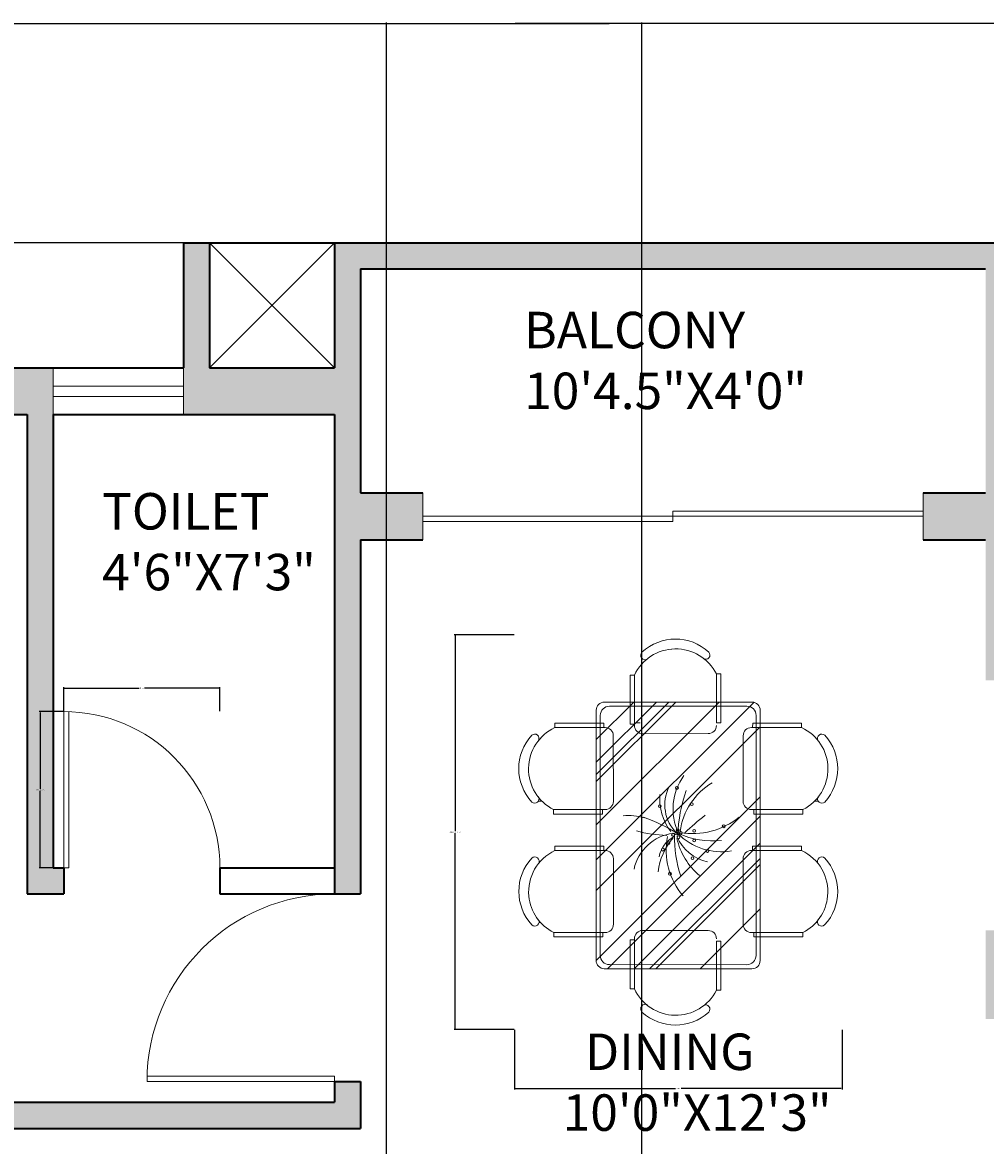
# Model space of a CAD drawing. Units: inches. Extents: x 2540 to 3167, y 3083 to 4007.
# Tile 13 of 15: x 2741 to 2926, y 3791 to 4007. Entities that reach past the tile are written whole.
import ezdxf

# ---------------------------------------------------------------- set-up
doc = ezdxf.new("R2010")
doc.units = ezdxf.units.IN
for name, color, linetype, lineweight in [('A-ANNO-DIMS', 2, 'Continuous', 18), ('A-AREA-IDEN', 7, 'Continuous', 18), ('A-DOOR', 4, 'Continuous', 18), ('A-FLOR-OPEN', 8, 'Continuous', 13), ('A-FURN', 8, 'Continuous', 13), ('A-GLAZ', 4, 'Continuous', 18)]:
    doc.layers.add(name, color=color, linetype=linetype, lineweight=lineweight)
doc.layers.add('A-WALL', color=143, linetype='Continuous', lineweight=35, true_color=0x7aafdf)
doc.layers.add('A-WALL-PATT', color=143, linetype='Continuous', lineweight=13, true_color=0x7aafdf)
doc.styles.get("Standard").update_dxf_attribs({"font": 'arial.ttf'})
doc.dimstyles.get("Standard").update_dxf_attribs({"dimtxt": 0.18, "dimasz": 0.18, "dimexe": 0.18, "dimexo": 0.0625, "dimgap": 0.09, "dimtad": 0, "dimtih": 1, "dimtoh": 1, "dimdec": 4, "dimzin": 0, "dimdsep": 46, "dimtxsty": 'Standard', "dimcen": 0.09, "dimadec": 0, "dimazin": 0, "dimtfac": 1, "dimtdec": 4, "dimtofl": 0, "dimtmove": 0, "dimatfit": 3, "dimfxl": 1, "dimtolj": 1, "dimtzin": 0, "dimarcsym": 0})

# ---------------------------------------------------------------- blocks, each defined once
blk = doc.blocks.new('A$C6327331B')
for p, q in [((790.8, 678.3), (790.8, 696.4)), ((790.8, 678.3), (790.8, 696.4)), ((1381.3, 692.8), (1381.3, 686.2)), ((1381.3, 692.8), (1381.3, 686.2)), ((410.1, 615.8), (410, 377)), ((410.1, 615.8), (410, 377)), ((431.6, 615.8), (410.1, 615.8)), ((431.6, 615.8), (410.1, 615.8)), ((431.4, 376.9), (431.6, 615.8)), ((431.4, 376.9), (431.6, 615.8)), ((831.4, 382.9), (831.6, 621.7)), ((831.4, 382.9), (831.6, 621.7)), ((831.6, 621.7), (853, 621.7)), ((831.6, 621.7), (853, 621.7)), ((853, 621.7), (852.9, 382.9)), ((853, 621.7), (852.9, 382.9)), ((1009.3, 615.5), (1009.2, 376.7)), ((1009.3, 615.5), (1009.2, 376.7)), ((1030.7, 615.5), (1009.3, 615.5)), ((1030.7, 615.5), (1009.3, 615.5)), ((1030.6, 376.6), (1030.7, 615.5)), ((1030.6, 376.6), (1030.7, 615.5)), ((1430.6, 382.6), (1430.7, 621.4)), ((1430.6, 382.6), (1430.7, 621.4)), ((1430.7, 621.4), (1452.2, 621.4)), ((1430.7, 621.4), (1452.2, 621.4)), ((1452.2, 621.4), (1452, 382.6)), ((1452.2, 621.4), (1452, 382.6)), ((431.5, 571.8), (431.4, 370.8)), ((431.5, 571.8), (431.4, 370.8)), ((831.4, 370.6), (831.5, 571.6)), ((831.4, 370.6), (831.5, 571.6)), ((1030.7, 571.5), (1030.6, 370.5)), ((1030.7, 571.5), (1030.6, 370.5)), ((1430.6, 370.3), (1430.7, 571.3)), ((1430.6, 370.3), (1430.7, 571.3)), ((347.5, 414), (831.5, 413.8)), ((347.5, 414), (831.5, 413.8)), ((372.5, 394), (831.4, 393.8)), ((372.5, 394), (1009.2, 393.7)), ((1226.3, -386.4), (428, 414)), ((1226.3, -386.4), (428, 414)), ((1567.1, -386.6), (768.8, 413.8)), ((1567.1, -386.6), (768.8, 413.8)), ((831.5, 413.8), (1567.5, 413.4)), ((1607.1, -331.3), (864.1, 413.8)), ((1607.1, -331.3), (864.1, 413.8)), ((1607.2, -200.8), (994.4, 413.7)), ((1607.2, -200.8), (994.4, 413.7)), ((1009.2, 413.7), (1567.5, 413.4)), ((1009.2, 393.7), (1542.5, 393.4)), ((1607.2, -125.5), (1069.5, 413.7)), ((1607.2, -125.5), (1069.5, 413.7)), ((1607.2, -95.4), (1099.6, 413.6)), ((1607.2, -95.4), (1099.6, 413.6)), ((1607.3, 120.5), (1315.1, 413.5)), ((1607.3, 120.5), (1315.1, 413.5)), ((1415.7, 413.4), (1415.7, 413.5)), ((1415.7, 413.4), (1415.7, 413.5)), ((307.1, -346), (307.5, 374)), ((307.1, -346), (307.5, 374)), ((1075.9, -386.3), (308.5, 383.1)), ((1075.9, -386.3), (308.5, 383.1)), ((327.1, -321), (327.5, 349)), ((410, 377), (431.4, 376.9)), ((410, 377), (431.4, 376.9)), ((471.4, 330.8), (791.4, 330.6)), ((471.4, 330.8), (791.4, 330.6)), ((852.9, 382.9), (831.4, 382.9)), ((852.9, 382.9), (831.4, 382.9)), ((1009.2, 376.7), (1030.6, 376.6)), ((1009.2, 376.7), (1030.6, 376.6)), ((1070.6, 330.5), (1390.6, 330.3)), ((1070.6, 330.5), (1390.6, 330.3)), ((1452, 382.6), (1430.6, 382.6)), ((1452, 382.6), (1430.6, 382.6)), ((1587.5, 348.4), (1587.1, -321.6)), ((1607.5, 373.4), (1607.1, -346.6)), ((1607.5, 373.4), (1607.1, -346.6)), ((169.9, 221.5), (408.7, 221.6)), ((169.9, 221.5), (408.7, 221.6)), ((169.9, 200.1), (169.9, 221.5)), ((169.9, 200.1), (169.9, 221.5)), ((408.7, 221.6), (408.7, 200.2)), ((408.7, 221.6), (408.7, 200.2)), ((1473.3, 221.6), (1473.3, 200.2)), ((1473.3, 221.6), (1473.3, 200.2)), ((1712.1, 221.5), (1473.3, 221.6)), ((1712.1, 221.5), (1473.3, 221.6)), ((1712.1, 200.1), (1712.1, 221.5)), ((1712.1, 200.1), (1712.1, 221.5)), ((408.7, 200.2), (169.9, 200.1)), ((408.7, 200.2), (169.9, 200.1)), ((905.5, -386.3), (307.4, 213.5)), ((905.5, -386.3), (307.4, 213.5)), ((1473.3, 200.2), (1712.1, 200.1)), ((1473.3, 200.2), (1712.1, 200.1)), ((461.2, -159.8), (461, 160.2)), ((461.2, -159.8), (461, 160.2)), ((1420.8, -159.8), (1420.9, 160.2)), ((1420.8, -159.8), (1420.9, 160.2)), ((695.1, -386.2), (307.3, 2.7)), ((695.1, -386.2), (307.3, 2.7)), ((44.6, -20.2), (44.5, -20.1)), ((44.6, -20.2), (44.5, -20.1)), ((660, -386.1), (307.3, -32.5)), ((660, -386.1), (307.3, -32.5)), ((1837.4, -20.2), (1837.5, -20.1)), ((1837.4, -20.2), (1837.5, -20.1)), ((599.8, -386.1), (307.2, -92.7)), ((599.8, -386.1), (307.2, -92.7)), ((415.1, -199.8), (176.2, -199.9)), ((415.1, -199.8), (176.2, -199.9)), ((176.2, -199.9), (176.2, -221.3)), ((176.2, -199.9), (176.2, -221.3)), ((220.2, -199.9), (421.2, -199.8)), ((220.2, -199.9), (421.2, -199.8)), ((489.6, -386), (307.2, -203.2)), ((489.6, -386), (307.2, -203.2)), ((408.7, -193.6), (408.7, -172.1)), ((408.7, -193.6), (408.7, -172.1)), ((415.1, -221.2), (415.1, -199.8)), ((415.1, -221.2), (415.1, -199.8)), ((1661.8, -199.9), (1460.8, -199.8)), ((1661.8, -199.9), (1460.8, -199.8)), ((1466.9, -221.2), (1466.9, -199.8)), ((1466.9, -221.2), (1466.9, -199.8)), ((1466.9, -199.8), (1705.7, -199.9)), ((1466.9, -199.8), (1705.7, -199.9)), ((1705.7, -199.9), (1705.7, -221.3)), ((1705.7, -199.9), (1705.7, -221.3)), ((176.2, -221.3), (415.1, -221.2)), ((176.2, -221.3), (415.1, -221.2)), ((1705.7, -221.3), (1466.9, -221.2)), ((1705.7, -221.3), (1466.9, -221.2)), ((471.4, -302.7), (791.4, -302.5)), ((471.4, -302.7), (791.4, -302.5)), ((1070.6, -302.4), (1390.6, -302.2)), ((1070.6, -302.4), (1390.6, -302.2)), ((1542.1, -366.6), (372.1, -366)), ((410.1, -587.7), (410, -348.9)), ((410.1, -587.7), (410, -348.9)), ((410, -348.9), (431.4, -348.9)), ((410, -348.9), (431.4, -348.9)), ((431.5, -543.7), (431.4, -342.7)), ((431.5, -543.7), (431.4, -342.7)), ((431.4, -348.9), (431.6, -587.7)), ((431.4, -348.9), (431.6, -587.7)), ((831.4, -342.5), (831.5, -543.5)), ((831.4, -342.5), (831.5, -543.5)), ((831.4, -354.8), (831.6, -593.6)), ((831.4, -354.8), (831.6, -593.6)), ((852.9, -354.8), (831.4, -354.8)), ((852.9, -354.8), (831.4, -354.8)), ((853, -593.6), (852.9, -354.8)), ((853, -593.6), (852.9, -354.8)), ((1009.2, -348.6), (1030.6, -348.5)), ((1009.2, -348.6), (1030.6, -348.5)), ((1009.3, -587.4), (1009.2, -348.6)), ((1009.3, -587.4), (1009.2, -348.6)), ((1030.7, -543.4), (1030.6, -342.4)), ((1030.7, -543.4), (1030.6, -342.4)), ((1030.6, -348.5), (1030.7, -587.4)), ((1030.6, -348.5), (1030.7, -587.4)), ((1430.6, -342.2), (1430.7, -543.2)), ((1430.6, -342.2), (1430.7, -543.2)), ((1430.6, -354.5), (1430.7, -593.3)), ((1430.6, -354.5), (1430.7, -593.3)), ((1452, -354.5), (1430.6, -354.5)), ((1452, -354.5), (1430.6, -354.5)), ((1452.2, -593.3), (1452, -354.5)), ((1452.2, -593.3), (1452, -354.5)), ((1567.1, -386.6), (347.1, -386)), ((1567.1, -386.6), (347.1, -386)), ((831.5, -385.7), (864.1, -385.7)), ((831.5, -385.7), (864.1, -385.7)), ((1415.7, -385.3), (1415.7, -385.4)), ((1415.7, -385.3), (1415.7, -385.4)), ((431.6, -587.7), (410.1, -587.7)), ((431.6, -587.7), (410.1, -587.7)), ((831.6, -593.6), (853, -593.6)), ((831.6, -593.6), (853, -593.6)), ((1030.7, -587.4), (1009.3, -587.4)), ((1030.7, -587.4), (1009.3, -587.4)), ((1430.7, -593.3), (1452.2, -593.3)), ((1430.7, -593.3), (1452.2, -593.3)), ((790.8, -650.2), (790.8, -668.4)), ((790.8, -650.2), (790.8, -668.4)), ((1381.3, -664.7), (1381.3, -658.1)), ((1381.3, -664.7), (1381.3, -658.1))]:
    blk.add_line(p, q)
for centre, radius, start, end in [((631.5, 550.5), 241.3, 47.4691, 132.4721), ((631.5, 550.5), 241.3, 47.4691, 132.4721), ((1230.7, 550.2), 241.3, 47.4691, 132.4721), ((1230.7, 550.2), 241.3, 47.4691, 132.4721), ((633, 521.6), 222.4, 26.7656, 154.9369), ((633, 521.6), 222.4, 26.7656, 154.9369), ((484.3, 714.2), 21.2, 137.6497, 300.3412), ((484.3, 714.2), 21.2, 137.6497, 300.3412), ((779, 714), 21.2, 239.6, 42.2915), ((779, 714), 21.2, 239.6, 42.2915), ((1232.2, 521.3), 222.4, 84.4265, 154.9369), ((1232.2, 521.3), 222.4, 84.4265, 154.9369), ((1083.4, 713.9), 21.2, 137.6497, 300.3412), ((1083.4, 713.9), 21.2, 137.6497, 300.3412), ((1232.2, 521.3), 222.4, 26.7656, 84.4265), ((1232.2, 521.3), 222.4, 26.7656, 84.4265), ((1378.1, 713.7), 21.2, 239.6, 42.2915), ((1378.1, 713.7), 21.2, 239.6, 42.2915), ((347.5, 374), 40, 89.9706, 179.9706), ((347.5, 374), 40, 89.9706, 179.9706), ((372.5, 349), 45, 89.9706, 179.9706), ((1542.5, 348.4), 45, 359.9706, 89.9706), ((1567.5, 373.4), 40, 359.9706, 89.9706), ((1567.5, 373.4), 40, 359.9706, 89.9706), ((471.4, 370.8), 40, 179.9706, 269.9706), ((471.4, 370.8), 40, 179.9706, 269.9706), ((791.4, 370.6), 40, 269.9706, 359.9706), ((791.4, 370.6), 40, 269.9706, 359.9706), ((1070.6, 370.5), 40, 179.9706, 269.9706), ((1070.6, 370.5), 40, 179.9706, 269.9706), ((1390.6, 370.3), 40, 269.9706, 359.9706), ((1390.6, 370.3), 40, 269.9706, 359.9706), ((574.1, 79.9), 374.6, 351.2496, 38.2333), ((912.6, 235.7), 6.91, 0, 180), ((912.6, 235.7), 6.91, 180, 0), ((737.8, 225), 299.2, 314.4861, 9.3762), ((586.4, 182.9), 398.1, 335.0888, 5.9637), ((270.2, 1.6), 222.4, 116.8244, 244.9957), ((270.2, 1.6), 222.4, 116.8244, 244.9957), ((77.6, 147.4), 21.2, 329.6588, 132.3503), ((77.6, 147.4), 21.2, 329.6588, 132.3503), ((421, 160.2), 40, 0.0294, 90.0294), ((421, 160.2), 40, 0.0294, 90.0294), ((983.2, 350.8), 331, 211.315, 262.1378), ((1460.9, 160.2), 40, 89.9706, 179.9706), ((1460.9, 160.2), 40, 89.9706, 179.9706), ((1611.7, 1.6), 222.4, 295.0043, 63.1756), ((1611.7, 1.6), 222.4, 295.0043, 63.1756), ((1804.4, 147.4), 21.2, 47.6497, 210.3412), ((1804.4, 147.4), 21.2, 47.6497, 210.3412), ((241.3, 0.1), 241.3, 137.5279, 222.5309), ((2460.3, 1443.6), 2062.1, 219.0488, 222.6799), ((873.8, 207.8), 219.3, 294.0956, 346.2953), ((897.1, 334.6), 335.6, 283.0452, 319.7766), ((1033, 155.9), 6.91, 0, 180), ((1033, 155.9), 6.91, 180, 0), ((1640.7, 0.1), 241.3, 317.4691, 42.4721), ((1640.7, 0.1), 241.3, 317.4691, 42.4721), ((805, 79.9), 6.91, 0, 180), ((805, 79.9), 6.91, 180, 0), ((934.8, 91.3), 6.91, 0, 180), ((934.8, 91.3), 6.91, 180, 0), ((982.3, 91.3), 6.91, 0, 180), ((982.3, 91.3), 6.91, 180, 0), ((1067.8, 83.7), 6.91, 0, 180), ((1067.8, 83.7), 6.91, 180, 0), ((826.9, 258.5), 270.1, 233.3231, 295.7633), ((725.8, 7.7), 6.91, 0, 180), ((725.8, 7.7), 6.91, 180, 0), ((807.8, 143), 194.5, 242.9909, 315.9102), ((985.1, 750.7), 739.8, 250.5249, 267.8244), ((1747.6, -469.5), 933.6, 148.9873, 160.361), ((931.7, 11.5), 6.91, 0, 180), ((931.7, 11.5), 6.91, 180, 0), ((944.3, 26.7), 6.91, 0, 180), ((944.3, 26.7), 6.91, 180, 0), ((947.5, 3.9), 6.91, 0, 180), ((947.5, 3.9), 6.91, 180, 0), ((970.7, 574.8), 578.8, 268.3286, 288.729), ((966.5, 15.3), 6.91, 0, 180), ((966.5, 15.3), 6.91, 180, 0), ((1030.3, 292.7), 337.4, 258.5516, 310.9815), ((776.7, 191.6), 268.2, 265.8741, 306.9558), ((392.7, -33), 564.4, 343.8561, 359.1105), ((953.8, -11.3), 6.91, 0, 180), ((953.8, -11.3), 6.91, 180, 0), ((1167.7, 15.7), 221.9, 186.9904, 258.0284), ((1090.6, 62.7), 145.4, 208.8901, 258.4579), ((1166.2, 212.9), 298.2, 228.7581, 263.8624), ((995, -34.1), 6.91, 0, 180), ((995, -34.1), 6.91, 180, 0), ((1026.7, -60.7), 6.91, 0, 180), ((1143.8, -26.5), 6.91, 0, 180), ((1143.8, -26.5), 6.91, 180, 0), ((814.5, -75.9), 6.91, 0, 180), ((814.5, -75.9), 6.91, 180, 0), ((1026.7, -60.7), 6.91, 180, 0), ((79, -146.7), 22.5, 226.3776, 29.8882), ((79, -146.7), 22.5, 226.3776, 29.8882), ((421.2, -159.8), 40, 270.0294, 0.0294), ((421.2, -159.8), 40, 270.0294, 0.0294), ((1112.9, -226), 252.6, 162.9456, 186.4814), ((1460.8, -159.8), 40, 179.9706, 269.9706), ((1460.8, -159.8), 40, 179.9706, 269.9706), ((1803, -146.7), 22.5, 150.1118, 313.6224), ((1803, -146.7), 22.5, 150.1118, 313.6224), ((372.1, -321), 45, 179.9706, 269.9706), ((471.4, -342.7), 40, 90.0294, 180.0294), ((471.4, -342.7), 40, 90.0294, 180.0294), ((791.4, -342.5), 40, 0.0294, 90.0294), ((791.4, -342.5), 40, 0.0294, 90.0294), ((1070.6, -342.4), 40, 90.0294, 180.0294), ((1070.6, -342.4), 40, 90.0294, 180.0294), ((1390.6, -342.2), 40, 0.0294, 90.0294), ((1390.6, -342.2), 40, 0.0294, 90.0294), ((1542.1, -321.6), 45, 269.9706, 359.9706), ((347.1, -346), 40, 179.9706, 269.9706), ((347.1, -346), 40, 179.9706, 269.9706), ((1567.1, -346.6), 40, 269.9706, 359.9706), ((1567.1, -346.6), 40, 269.9706, 359.9706), ((633, -493.5), 222.4, 205.0631, 333.2344), ((633, -493.5), 222.4, 205.0631, 333.2344), ((1232.2, -493.2), 222.4, 205.0631, 275.5735), ((1232.2, -493.2), 222.4, 205.0631, 275.5735), ((1232.2, -493.2), 222.4, 275.5735, 333.2344), ((1232.2, -493.2), 222.4, 275.5735, 333.2344), ((484.3, -686.1), 21.2, 59.6588, 222.3503), ((484.3, -686.1), 21.2, 59.6588, 222.3503), ((631.5, -522.4), 241.3, 227.5279, 312.5309), ((631.5, -522.4), 241.3, 227.5279, 312.5309), ((779, -686), 21.2, 317.7085, 120.4), ((779, -686), 21.2, 317.7085, 120.4), ((1083.4, -685.8), 21.2, 59.6588, 222.3503), ((1083.4, -685.8), 21.2, 59.6588, 222.3503), ((1230.7, -522.1), 241.3, 227.5279, 312.5309), ((1230.7, -522.1), 241.3, 227.5279, 312.5309), ((1378.1, -685.6), 21.2, 317.7085, 120.4), ((1378.1, -685.6), 21.2, 317.7085, 120.4)]:
    blk.add_arc(centre, radius, start, end)
at = {"width": 0.8, "flags": 9}
for tag in ['XSIZE', 'YSIZE']:
    blk.add_attdef(tag, (945.2, 11.4), '', height=0.23, rotation=180, dxfattribs=at)
blk = doc.blocks.new('DOOR-SWING-36IN')
for p, q in [((36, 0), (0, 0)), ((36, 1), (0.01, 1)), ((36, 1), (36, 0))]:
    blk.add_line(p, q)
blk.add_arc((36, 0), 36, 90, 180)
blk = doc.blocks.new('DOOR-SWING-30IN')
for p, q in [((0, 0), (0, 30)), ((1, 0), (1, 29.98)), ((0, 0), (1, 0))]:
    blk.add_line(p, q)
blk.add_arc((0, 0), 30, 0, 90)
blk = doc.blocks.new('OPENING-CROSS-24IN')
for p, q in [((24, 24), (0, 0)), ((0, 24), (24, 0))]:
    blk.add_line(p, q)
blk = doc.blocks.new('*D21')
at = {"layer": 'A-ANNO-DIMS', "color": 0, "lineweight": -2, "transparency": 16777216}
for p, q in [((2748.45, 3874.71), (2743.83, 3874.71)), ((2744.01, 3874.53), (2744.01, 3859.9)), ((2744.01, 3844.89), (2744.01, 3859.53)), ((2748.45, 3844.71), (2743.83, 3844.71))]:
    blk.add_line(p, q, dxfattribs=at)
at = {"layer": 'A-ANNO-DIMS', "color": 0, "transparency": 16777216}
for points in [[(2743.98, 3874.53), (2744.04, 3874.53), (2744.01, 3874.71)], [(2743.98, 3844.89), (2744.04, 3844.89), (2744.01, 3844.71)]]:
    blk.add_solid(points, dxfattribs=at)
at = {"layer": 'Defpoints', "color": 0, "transparency": 16777216}
for p in [(2744.01, 3874.71), (2748.51, 3874.71), (2748.51, 3844.71)]:
    blk.add_point(p, dxfattribs=at)
at = {"layer": 'A-ANNO-DIMS', "color": 0, "transparency": 16777216, "insert": (2744.01, 3859.71), "char_height": 0.18, "attachment_point": 5}
blk.add_mtext('\\A1;DOOR 30 TYP.', dxfattribs=at)
blk = doc.blocks.new('*D22')
at = {"layer": 'A-ANNO-DIMS', "color": 0, "lineweight": -2, "transparency": 16777216}
for p, q in [((2748.51, 3874.78), (2748.51, 3879.39)), ((2748.69, 3879.21), (2762.98, 3879.21)), ((2778.33, 3879.21), (2764.04, 3879.21)), ((2778.51, 3874.78), (2778.51, 3879.39))]:
    blk.add_line(p, q, dxfattribs=at)
at = {"layer": 'A-ANNO-DIMS', "color": 0, "transparency": 16777216}
for points in [[(2748.69, 3879.24), (2748.69, 3879.18), (2748.51, 3879.21)], [(2778.33, 3879.24), (2778.33, 3879.18), (2778.51, 3879.21)]]:
    blk.add_solid(points, dxfattribs=at)
at = {"layer": 'Defpoints', "color": 0, "transparency": 16777216}
for p in [(2778.51, 3879.21), (2748.51, 3874.71), (2778.51, 3874.71)]:
    blk.add_point(p, dxfattribs=at)
at = {"layer": 'A-ANNO-DIMS', "color": 0, "transparency": 16777216, "insert": (2763.51, 3879.21), "char_height": 0.18, "attachment_point": 5}
blk.add_mtext('\\A1;30 TYP.', dxfattribs=at)
blk = doc.blocks.new('*D37')
at = {"layer": 'A-ANNO-DIMS', "color": 0, "lineweight": -2, "transparency": 16777216}
for p, q in [((2834.99, 3889.47), (2823.51, 3889.47)), ((2823.69, 3889.29), (2823.69, 3851.77)), ((2823.69, 3813.89), (2823.69, 3851.4)), ((2834.99, 3813.71), (2823.51, 3813.71))]:
    blk.add_line(p, q, dxfattribs=at)
at = {"layer": 'A-ANNO-DIMS', "color": 0, "transparency": 16777216}
for points in [[(2823.66, 3889.29), (2823.72, 3889.29), (2823.69, 3889.47)], [(2823.66, 3813.89), (2823.72, 3813.89), (2823.69, 3813.71)]]:
    blk.add_solid(points, dxfattribs=at)
at = {"layer": 'Defpoints', "color": 0, "transparency": 16777216}
for p in [(2835.06, 3889.47), (2823.69, 3813.71), (2835.06, 3813.71)]:
    blk.add_point(p, dxfattribs=at)
at = {"layer": 'A-ANNO-DIMS', "color": 0, "transparency": 16777216, "insert": (2823.69, 3851.59), "char_height": 0.18, "attachment_point": 5}
blk.add_mtext('\\A1;DINING SET 76 TYP.', dxfattribs=at)
blk = doc.blocks.new('*D38')
at = {"layer": 'A-ANNO-DIMS', "color": 0, "lineweight": -2, "transparency": 16777216}
for p, q in [((2835.06, 3813.64), (2835.06, 3802.16)), ((2897.96, 3813.64), (2897.96, 3802.16)), ((2835.24, 3802.34), (2865.98, 3802.34)), ((2897.78, 3802.34), (2867.04, 3802.34))]:
    blk.add_line(p, q, dxfattribs=at)
at = {"layer": 'A-ANNO-DIMS', "color": 0, "transparency": 16777216}
for points in [[(2835.24, 3802.37), (2835.24, 3802.31), (2835.06, 3802.34)], [(2897.78, 3802.37), (2897.78, 3802.31), (2897.96, 3802.34)]]:
    blk.add_solid(points, dxfattribs=at)
at = {"layer": 'Defpoints', "color": 0, "transparency": 16777216}
for p in [(2835.06, 3813.71), (2897.96, 3813.71), (2897.96, 3802.34)]:
    blk.add_point(p, dxfattribs=at)
at = {"layer": 'A-ANNO-DIMS', "color": 0, "transparency": 16777216, "insert": (2866.51, 3802.34), "char_height": 0.18, "attachment_point": 5}
blk.add_mtext('\\A1;63 TYP.', dxfattribs=at)
blk = doc.blocks.new('*D43')
at = {"layer": 'A-ANNO-DIMS', "color": 0, "lineweight": -2, "transparency": 16777216}
for p, q in [((2582.51, 3940.78), (2582.51, 4006.99)), ((2582.69, 4006.81), (2853.22, 4006.81)), ((3124.33, 4006.81), (2853.8, 4006.81)), ((3124.51, 3940.78), (3124.51, 4006.99))]:
    blk.add_line(p, q, dxfattribs=at)
at = {"layer": 'A-ANNO-DIMS', "color": 0, "transparency": 16777216}
for points in [[(2582.69, 4006.84), (2582.69, 4006.78), (2582.51, 4006.81)], [(3124.33, 4006.84), (3124.33, 4006.78), (3124.51, 4006.81)]]:
    blk.add_solid(points, dxfattribs=at)
at = {"layer": 'Defpoints', "color": 0, "transparency": 16777216}
for p in [(3124.51, 4006.81), (2582.51, 3940.71), (3124.51, 3940.71)]:
    blk.add_point(p, dxfattribs=at)
at = {"layer": 'A-ANNO-DIMS', "color": 0, "transparency": 16777216, "insert": (2853.51, 4006.81), "char_height": 0.18, "attachment_point": 5}
blk.add_mtext('\\A1;542', dxfattribs=at)
blk = doc.blocks.new('*D44')
at = {"layer": 'A-ANNO-DIMS', "color": 0, "lineweight": -2, "transparency": 16777216}
for p, q in [((2771.45, 3964.71), (2540.23, 3964.71)), ((2540.41, 3964.53), (2540.41, 3545.4)), ((2540.41, 3125.89), (2540.41, 3545.03)), ((2810.45, 3125.71), (2540.23, 3125.71))]:
    blk.add_line(p, q, dxfattribs=at)
at = {"layer": 'A-ANNO-DIMS', "color": 0, "transparency": 16777216}
for points in [[(2540.38, 3964.53), (2540.44, 3964.53), (2540.41, 3964.71)], [(2540.38, 3125.89), (2540.44, 3125.89), (2540.41, 3125.71)]]:
    blk.add_solid(points, dxfattribs=at)
at = {"layer": 'Defpoints', "color": 0, "transparency": 16777216}
for p in [(2540.41, 3964.71), (2771.51, 3964.71), (2810.51, 3125.71)]:
    blk.add_point(p, dxfattribs=at)
at = {"layer": 'A-ANNO-DIMS', "color": 0, "transparency": 16777216, "insert": (2540.41, 3545.21), "char_height": 0.18, "attachment_point": 5}
blk.add_mtext('\\A1;839', dxfattribs=at)
blk = doc.blocks.new('*D56')
at = {"layer": 'A-ANNO-DIMS', "color": 0, "lineweight": -2, "transparency": 16777216}
for p, q in [((2810.51, 3564.78), (2810.51, 4006.99)), ((2810.69, 4006.81), (2834.79, 4006.81)), ((2859.33, 4006.81), (2835.23, 4006.81)), ((2859.51, 3564.78), (2859.51, 4006.99))]:
    blk.add_line(p, q, dxfattribs=at)
at = {"layer": 'A-ANNO-DIMS', "color": 0, "transparency": 16777216}
for points in [[(2810.69, 4006.84), (2810.69, 4006.78), (2810.51, 4006.81)], [(2859.33, 4006.84), (2859.33, 4006.78), (2859.51, 4006.81)]]:
    blk.add_solid(points, dxfattribs=at)
at = {"layer": 'Defpoints', "color": 0, "transparency": 16777216}
for p in [(2859.51, 4006.81), (2810.51, 3564.71), (2859.51, 3564.71)]:
    blk.add_point(p, dxfattribs=at)
at = {"layer": 'A-ANNO-DIMS', "color": 0, "transparency": 16777216, "insert": (2835.01, 4006.81), "char_height": 0.18, "attachment_point": 5}
blk.add_mtext('\\A1;49', dxfattribs=at)

msp = doc.modelspace()

# ---------------------------------------------------------------- hatches: boundary and pattern name
at = {"layer": 'A-WALL-PATT'}
h = msp.add_hatch(color=256, dxfattribs=at)
h.dxf.hatch_style = 1
h.paths.add_polyline_path([(2644.77, 3940.71), (2582.51, 3940.71), (2582.51, 3886.71), (2612.51, 3886.71), (2612.51, 3871.71), (2621.51, 3871.71), (2621.51, 3895.71), (2591.51, 3895.71), (2591.51, 3931.71), (2621.51, 3931.71), (2644.77, 3931.71)])
h.paths.add_polyline_path([(2746.51, 3940.71), (2716.77, 3940.71), (2716.77, 3931.71), (2741.51, 3931.71), (2741.51, 3839.71), (2748.51, 3839.71), (2748.51, 3844.71), (2746.51, 3844.71), (2746.51, 3931.71)])
h.paths.add_polyline_path([(2805.51, 3959.71), (2925.51, 3959.71), (2925.51, 3916.71), (2913.51, 3916.71), (2913.51, 3907.71), (2925.51, 3907.71), (2925.51, 3880.71), (2930.51, 3880.71), (2930.51, 3931.71), (2978.28, 3931.71), (2978.28, 3940.71), (2930.51, 3940.71), (2930.51, 3964.71), (2800.51, 3964.71), (2800.51, 3940.71), (2776.51, 3940.71), (2776.51, 3964.71), (2771.51, 3964.71), (2771.51, 3940.71), (2771.51, 3931.71), (2800.51, 3931.71), (2800.51, 3839.71), (2805.51, 3839.71), (2805.51, 3907.71), (2817.48, 3907.71), (2817.48, 3916.71), (2805.51, 3916.71)])
h.paths.add_polyline_path([(3124.51, 3940.71), (3026.28, 3940.71), (3026.28, 3931.71), (3062.51, 3931.71), (3062.51, 3924.21), (3071.51, 3924.21), (3071.51, 3931.71), (3119.51, 3931.71), (3119.51, 3832.71), (2925.51, 3832.71), (2925.51, 3815.71), (2930.51, 3815.71), (2930.51, 3827.71), (2976.51, 3827.71), (2976.51, 3773.71), (2970.51, 3773.71), (2970.51, 3768.71), (2985.51, 3768.71), (2985.51, 3773.71), (2981.51, 3773.71), (2981.51, 3827.71), (3086.51, 3827.71), (3086.51, 3812.71), (3095.51, 3812.71), (3095.51, 3827.71), (3124.51, 3827.71)])
h = msp.add_hatch(color=256, dxfattribs=at)
h.dxf.hatch_style = 1
h.paths.add_polyline_path([(2805.51, 3803.71), (2800.51, 3803.71), (2800.51, 3799.71), (2621.51, 3799.71), (2621.51, 3823.71), (2612.51, 3823.71), (2612.51, 3794.71), (2636.51, 3794.71), (2636.51, 3782.71), (2645.51, 3782.71), (2645.51, 3794.71), (2805.51, 3794.71)])
h.paths.add_polyline_path([(2810.51, 3564.71), (2868.51, 3564.71), (2868.51, 3627.71), (2872.51, 3627.71), (2872.51, 3636.71), (2864.51, 3636.71), (2864.51, 3674.71), (2797.51, 3674.71), (2797.51, 3669.71), (2801.51, 3669.71), (2801.51, 3628.63), (2806.51, 3628.63), (2806.51, 3669.71), (2859.51, 3669.71), (2859.51, 3573.71), (2806.51, 3573.71), (2806.51, 3598.63), (2801.51, 3598.63), (2801.51, 3549.71), (2645.51, 3549.71), (2645.51, 3573.71), (2636.51, 3573.71), (2636.51, 3516.71), (2645.51, 3516.71), (2645.51, 3540.71), (2801.51, 3540.71), (2801.51, 3504.71), (2801.51, 3500.71), (2806.51, 3500.71), (2806.51, 3504.71), (2859.51, 3504.71), (2859.51, 3420.71), (2806.51, 3420.71), (2806.51, 3470.71), (2801.51, 3470.71), (2801.51, 3420.71), (2797.51, 3420.71), (2797.51, 3415.71), (2864.51, 3415.71), (2864.51, 3453.71), (2868.51, 3453.71), (2868.51, 3513.71), (2810.51, 3513.71)])
h.paths.add_polyline_path([(2645.51, 3415.71), (2761.51, 3415.71), (2761.51, 3420.71), (2645.51, 3420.71), (2645.51, 3444.71), (2636.51, 3444.71), (2636.51, 3403.71), (2645.51, 3403.71)])
h.paths.add_polyline_path([(2645.51, 3307.71), (2636.51, 3307.71), (2636.51, 3295.71), (2612.51, 3295.71), (2612.51, 3149.71), (2645.51, 3149.71), (2645.51, 3158.71), (2621.51, 3158.71), (2621.51, 3290.71), (2801.51, 3290.71), (2801.51, 3286.71), (2806.51, 3286.71), (2806.51, 3295.71), (2645.51, 3295.71)])
h.paths.add_polyline_path([(2762.01, 3158.71), (2746.51, 3158.71), (2746.51, 3240.71), (2750.51, 3240.71), (2750.51, 3245.71), (2741.51, 3245.71), (2741.51, 3158.71), (2717.51, 3158.71), (2717.51, 3149.71), (2762.01, 3149.71)], flags=17)
h.paths.add_polyline_path([(2810.51, 3173.71), (2822.51, 3173.71), (2822.51, 3182.71), (2806.51, 3182.71), (2806.51, 3250.71), (2801.51, 3250.71), (2801.51, 3245.71), (2780.51, 3245.71), (2780.51, 3240.71), (2801.51, 3240.71), (2801.51, 3158.71), (2786.01, 3158.71), (2786.01, 3149.71), (2810.51, 3149.71)])
h.paths.add_polyline_path([(2931.51, 3290.71), (2935.51, 3290.71), (2935.51, 3295.71), (2926.51, 3295.71), (2926.51, 3182.71), (2910.51, 3182.71), (2910.51, 3173.71), (2922.51, 3173.71), (2922.51, 3149.71), (2987.51, 3149.71), (2987.51, 3158.71), (2931.51, 3158.71)])
h.paths.add_polyline_path([(3124.51, 3295.71), (3086.51, 3295.71), (3018.51, 3295.71), (3018.51, 3290.71), (3115.51, 3290.71), (3115.51, 3158.71), (3059.51, 3158.71), (3059.51, 3149.71), (3124.51, 3149.71)])
h.paths.add_polyline_path([(2988.51, 3295.71), (2984.51, 3295.71), (2984.51, 3349.71), (3086.51, 3349.71), (3086.51, 3320.71), (3124.51, 3320.71), (3124.51, 3354.71), (3071.51, 3354.71), (3071.51, 3358.71), (3062.51, 3358.71), (3062.51, 3354.71), (2979.51, 3354.71), (2979.51, 3295.71), (2971.51, 3295.71), (2971.51, 3290.71), (2988.51, 3290.71)])
h.paths.add_polyline_path([(3095.51, 3325.71), (3095.51, 3349.71), (3119.51, 3349.71), (3119.51, 3325.71)], flags=16)
h.paths.add_polyline_path([(3124.51, 3462.71), (3071.51, 3462.71), (3071.51, 3627.71), (3124.51, 3627.71), (3124.51, 3693.71), (3095.51, 3693.71), (3095.51, 3702.71), (3086.51, 3702.71), (3086.51, 3684.71), (3086.51, 3636.71), (2930.51, 3636.71), (2930.51, 3768.71), (2934.51, 3768.71), (2934.51, 3773.71), (2930.51, 3773.71), (2925.51, 3773.71), (2925.51, 3730.71), (2864.51, 3730.71), (2864.51, 3760.71), (2859.51, 3760.71), (2859.51, 3725.71), (2925.51, 3725.71), (2925.51, 3636.71), (2908.51, 3636.71), (2908.51, 3627.71), (3062.51, 3627.71), (3062.51, 3543.71), (2930.51, 3543.71), (2930.51, 3534.71), (2993.51, 3534.71), (2993.51, 3516.71), (3002.51, 3516.71), (3002.51, 3534.71), (3062.51, 3534.71), (3062.51, 3462.71), (3002.51, 3462.71), (3002.51, 3480.71), (2993.51, 3480.71), (2993.51, 3462.71), (2916.51, 3462.71), (2916.51, 3453.71), (2926.51, 3453.71), (2926.51, 3361.71), (2859.51, 3361.71), (2859.51, 3338.71), (2864.51, 3338.71), (2864.51, 3356.71), (2926.51, 3356.71), (2926.51, 3338.71), (2931.51, 3338.71), (2931.51, 3453.71), (3062.51, 3453.71), (3062.51, 3448.21), (3071.51, 3448.21), (3071.51, 3453.71), (3124.51, 3453.71)])

# ---------------------------------------------------------------- linework, layer by layer
at = {"layer": 'A-DOOR'}
for p, q in [((2817.48, 3907.71), (2817.48, 3916.71)), ((2913.51, 3916.71), (2913.51, 3907.71)), ((2913.51, 3913.21), (2865.5, 3913.21)), ((2865.5, 3911.21), (2865.5, 3913.21)), ((2913.51, 3912.21), (2817.48, 3912.21)), ((2865.5, 3911.21), (2817.48, 3911.21))]:
    msp.add_line(p, q, dxfattribs=at)
at = {"layer": 'A-GLAZ'}
for p, q in [((2746.51, 3931.71), (2746.51, 3940.71)), ((2771.51, 3940.71), (2771.51, 3931.71)), ((2771.51, 3937.21), (2746.51, 3937.21)), ((2771.51, 3935.21), (2746.51, 3935.21))]:
    msp.add_line(p, q, dxfattribs=at)
at = {"layer": 'A-WALL'}
for p, q in [((2771.51, 3964.71), (2771.51, 3940.71)), ((2771.51, 3964.71), (2800.51, 3964.71)), ((2776.51, 3964.71), (2776.51, 3940.71)), ((2800.51, 3964.71), (2800.51, 3940.71)), ((2800.51, 3964.71), (2930.51, 3964.71)), ((2805.51, 3959.71), (2805.51, 3916.71)), ((2805.51, 3959.71), (2925.51, 3959.71)), ((2582.51, 3940.71), (2771.51, 3940.71)), ((2776.51, 3940.71), (2800.51, 3940.71)), ((2591.51, 3931.71), (2741.51, 3931.71)), ((2741.51, 3931.71), (2741.51, 3839.71)), ((2746.51, 3931.71), (2746.51, 3844.71)), ((2746.51, 3931.71), (2800.51, 3931.71)), ((2800.51, 3931.71), (2800.51, 3839.71)), ((2805.51, 3916.71), (2817.48, 3916.71)), ((2913.51, 3916.71), (2925.51, 3916.71)), ((2805.51, 3907.71), (2817.48, 3907.71)), ((2805.51, 3907.71), (2805.51, 3839.71)), ((2913.51, 3907.71), (2925.51, 3907.71)), ((2746.51, 3844.71), (2748.51, 3844.71)), ((2748.51, 3844.71), (2748.51, 3839.71)), ((2778.51, 3844.71), (2778.51, 3839.71)), ((2778.51, 3844.71), (2800.51, 3844.71)), ((2741.51, 3839.71), (2748.51, 3839.71)), ((2778.51, 3839.71), (2805.51, 3839.71)), ((2800.51, 3803.71), (2805.51, 3803.71)), ((2800.51, 3803.71), (2800.51, 3799.71)), ((2805.51, 3803.71), (2805.51, 3794.71)), ((2621.51, 3799.71), (2800.51, 3799.71)), ((2645.51, 3794.71), (2805.51, 3794.71))]:
    msp.add_line(p, q, dxfattribs=at)

# ---------------------------------------------------------------- block references
at = {"layer": 'A-DOOR'}
for name, p in [('DOOR-SWING-30IN', (2748.51, 3844.71)), ('DOOR-SWING-36IN', (2764.51, 3803.71))]:
    msp.add_blockref(name, p, dxfattribs=at)
at = {"layer": 'A-FLOR-OPEN'}
msp.add_blockref('OPENING-CROSS-24IN', (2776.51, 3940.71), dxfattribs=at)
at = {"layer": 'A-FURN', "xscale": 0.0393700787401575, "yscale": 0.0393700787401575, "zscale": 0.0393700787401575, "rotation": 270}
msp.add_blockref('A$C6327331B', (2865.96, 3888.63), dxfattribs=at)

# ---------------------------------------------------------------- texts
at = {"layer": 'A-AREA-IDEN', "char_height": 7, "attachment_point": 1}
for s, width, insert in [('BALCONY\\P10\'4.5"X4\'0"', 97.3161, (2836.92, 3951.45)), ('TOILET\\P4\'6"X7\'3"', 40.7219, (2755.89, 3916.66)), ('  DINING\\P10\'0"X12\'3"', 75.7339, (2844.32, 3812.91))]:
    msp.add_mtext_dynamic_manual_height_columns(s, width=width, gutter_width=12.5, heights=[0], dxfattribs=dict(at, insert=insert))

# ---------------------------------------------------------------- dimensions: what is measured, and where the dimension line sits
at = {"layer": 'A-ANNO-DIMS'}
for base, p1, p2, picture, middle in [((3124.51, 4006.81), (2582.51, 3940.71), (3124.51, 3940.71), '*D43', (2853.51, 4006.81)), ((2859.51, 4006.81), (2810.51, 3564.71), (2859.51, 3564.71), '*D56', (2835.01, 4006.81))]:
    dim = msp.add_linear_dim(base=base, p1=p1, p2=p2, dimstyle='Standard', override={"dimdec": 0, "dimlfac": 1, "dimrnd": 0, "dimzin": 0, "dimdsep": 46, "dimlunit": 2}, dxfattribs=at)
    dim.commit()
    dim.dimension.update_dxf_attribs({"geometry": picture, "text_midpoint": middle})
dim = msp.add_linear_dim(base=(2540.41, 3964.71), p1=(2810.51, 3125.71), p2=(2771.51, 3964.71), angle=90, dimstyle='Standard', override={"dimdec": 0, "dimlfac": 1, "dimrnd": 0, "dimzin": 0, "dimdsep": 46, "dimlunit": 2}, dxfattribs=at)
dim.commit()
dim.dimension.update_dxf_attribs({"geometry": '*D44', "text_midpoint": (2540.41, 3545.21)})
for base, p1, p2, angle, text, picture, middle in [((2823.69, 3813.71), (2835.06, 3889.47), (2835.06, 3813.71), 270, 'DINING SET <> TYP.', '*D37', (2823.69, 3851.59)), ((2744.01, 3874.71), (2748.51, 3844.71), (2748.51, 3874.71), 90, 'DOOR <> TYP.', '*D21', (2744.01, 3859.71))]:
    dim = msp.add_linear_dim(base=base, p1=p1, p2=p2, angle=angle, text=text, dimstyle='Standard', override={"dimdec": 0, "dimlfac": 1, "dimrnd": 0, "dimzin": 0, "dimdsep": 46, "dimlunit": 2}, dxfattribs=at)
    dim.commit()
    dim.dimension.update_dxf_attribs({"geometry": picture, "text_midpoint": middle})
for base, p1, p2, picture, middle in [((2778.51, 3879.21), (2748.51, 3874.71), (2778.51, 3874.71), '*D22', (2763.51, 3879.21)), ((2897.96, 3802.34), (2835.06, 3813.71), (2897.96, 3813.71), '*D38', (2866.51, 3802.34))]:
    dim = msp.add_linear_dim(base=base, p1=p1, p2=p2, text='<> TYP.', dimstyle='Standard', override={"dimdec": 0, "dimlfac": 1, "dimrnd": 0, "dimzin": 0, "dimdsep": 46, "dimlunit": 2}, dxfattribs=at)
    dim.commit()
    dim.dimension.update_dxf_attribs({"geometry": picture, "text_midpoint": middle})

doc.saveas('drawing.dxf')
